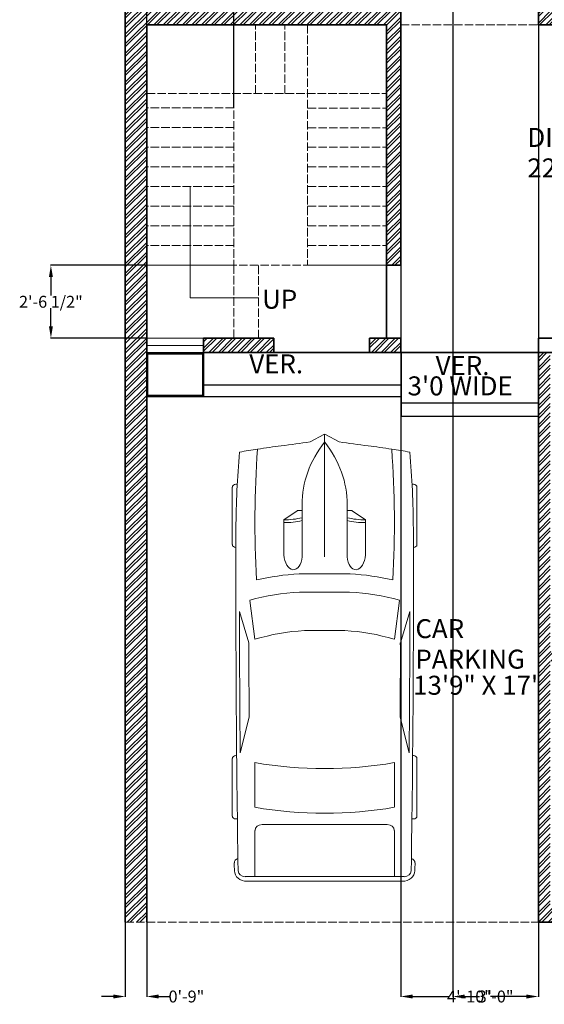
# Model space of a CAD drawing. Units: inches. Extents: x 334 to 846, y -424 to 250.
# Tile 1 of 3: x 336 to 557, y -420 to -5. Entities that reach past the tile are written whole.
import ezdxf

# ---------------------------------------------------------------- set-up
doc = ezdxf.new("R2010")
doc.units = ezdxf.units.IN
doc.header["$MEASUREMENT"] = 0
doc.linetypes.add('ACAD_ISO02W100', pattern=[15, 12, -3])
for name, color, linetype, lineweight in [('A-ANNO-SYMB', 7, 'Continuous', 18), ('A-ANNO-TEXT', 130, 'Continuous', 18), ('A-AREA-IDEN', 130, 'Continuous', 18), ('A-FLOR', 7, 'Continuous', 25), ('A-FLOR-STRS', 7, 'ACAD_ISO02W100', 18), ('A-WALL', 7, 'Continuous', 35), ('A-WALL-OVHD', 8, 'ACAD_ISO02W100', 18), ('A-WALL-PATT', 252, 'Continuous', 13), ('C-PRKG-VEHC', 8, 'Continuous', 18), ('C-PROP', 7, 'ACAD_ISO02W100', 18), ('dimension', 130, 'Continuous', 18), ('window', 150, 'Continuous', 18)]:
    doc.layers.add(name, color=color, linetype=linetype, lineweight=lineweight)
doc.styles.get("Standard").update_dxf_attribs({"font": 'arial.ttf'})
doc.dimstyles.get("Standard").update_dxf_attribs({"dimtxt": 5, "dimasz": 5, "dimexe": 0.18, "dimexo": 0.0625, "dimgap": 0.09, "dimtad": 0, "dimtih": 1, "dimtoh": 1, "dimdec": 1, "dimzin": 0, "dimdsep": 46, "dimlunit": 4, "dimtxsty": 'Standard', "dimcen": 0.09, "dimadec": 0, "dimazin": 0, "dimtfac": 1, "dimtdec": 1, "dimtofl": 0, "dimtmove": 0, "dimatfit": 3, "dimfxl": 1, "dimtolj": 1, "dimtzin": 0, "dimarcsym": 0})

# ---------------------------------------------------------------- blocks, each defined once
blk = doc.blocks.new('*U6')
for p, q in [((536, 950), (536, 936)), ((1182, 988), (568, 988)), ((1214, 950), (1214, 950)), ((3440, 942), (3440, 950)), ((3472, 988), (4087, 988)), ((4119, 950), (4119, 934)), ((2235, 810), (1899, 912)), ((3412, 904), (3030, 807)), ((4736, -851), (4736, 851)), ((1779, 801), (2195, 746)), ((3516, 746), (3994, 746)), ((4736, 746), (4242, 746)), ((4785, -832), (4785, 832)), ((4179, 670), (4179, -670)), ((820, 295), (918, 436)), ((918, 436), (1294, 436)), ((756, 241), (1313, 241)), ((816, 241), (816, 283)), ((1496, -274), (1496, 274)), ((1690, -267), (1690, 267)), ((2102, 216), (2102, -216)), ((4736, -267), (4736, 267)), ((83, 156), (3, 10)), ((0, 0), (1313, 0)), ((3, -10), (83, -156)), ((756, -241), (1313, -241)), ((816, -241), (816, -283)), ((820, -295), (918, -436)), ((918, -436), (1294, -436)), ((2195, -746), (1779, -801)), ((2235, -810), (1899, -912)), ((3412, -904), (3030, -807)), ((3994, -746), (3516, -746)), ((4242, -746), (4736, -746)), ((536, -950), (536, -936)), ((3440, -942), (3440, -950)), ((4119, -950), (4119, -934)), ((1182, -988), (568, -988)), ((1214, -950), (1214, -950)), ((3472, -988), (4087, -988))]:
    blk.add_line(p, q)
for centre, major_axis, ratio, start_param, end_param in [((1046, -12468), (0, 13417), 0.842304, 0.00281, 0.075598), ((568, 950), (0, -37.6), 0.842304, 3.141593, 4.712389), ((1638, -268113), (0, 269063), 0.842304, -0.013397, 0.002797), ((1182, 950), (0, 37.6), 0.842304, -1.570796, 0), ((3472, 950), (0, -37.6), 0.842304, 3.141593, 4.712389), ((4087, 950), (0, 37.6), 0.842304, -1.570796, 0), ((4588, 910), (0, 56.4), 0.842304, -0.013017, 1.249894), ((1638, -268131), (0, 269121), 0.842304, -0.013397, -0.013017), ((4673, 832), (0, -133), 0.842304, 1.570796, 3.128196), ((6757, -699), (0, 7958), 0.842304, 1.367076, 1.39176), ((1638, -268113), (0, -269025), 0.842304, 3.133765, 3.140441), ((4673, 851), (0, -75.2), 0.842304, 1.570796, 3.128196), ((952, -15087), (0, -15833), 0.842304, 3.096046, 3.200911), ((3436, 137), (0, 2077), 0.842304, 1.245306, 1.50788), ((3800, 71), (0, -2021), 0.842304, 4.372215, 4.640744), ((2433, -93125), (0, -93935), 0.842304, 3.134049, 3.144098), ((434, 0), (0, 3734), 0.842304, 4.511394, 4.913384), ((912, 0), (0, 3734), 0.842304, 4.511394, 4.913384), ((4242, 670), (0, 75.2), 0.842304, 0, 1.570796), ((6583, -699), (0, -7755), 0.842304, 4.528606, 4.561838), ((3414, 137), (0, -2280), 0.842304, 4.449482, 4.652344), ((-5194, 1331), (0, -6374), 0.842304, 1.385369, 1.434372), ((331, 432), (0, 696), 0.842304, 4.435146, 4.718221), ((361, 432), (0, 696), 0.842304, 4.435146, 4.718221), ((1290, 339), (161, -9), 0.603834, -1.395552, 1.581315), ((756, -1185), (0, 1427), 0.842304, 0, 0.590319), ((832, 283), (0, 18.8), 0.842304, 0.879714, 1.570796), ((16, 0), (0, -18.8), 0.842304, 4.131459, 5.293319), ((756, 1185), (0, 1427), 0.842304, 2.551274, 3.141593), ((-5194, -1331), (0, 6374), 0.842304, -1.434372, -1.385369), ((832, -283), (0, -18.8), 0.842304, 4.712389, 5.403472), ((331, -432), (0, -696), 0.842304, 1.564964, 1.848039), ((361, -432), (0, -696), 0.842304, 1.564964, 1.848039), ((3414, -137), (0, -2280), 0.842304, -1.510751, -1.307889), ((3436, -137), (0, -2077), 0.842304, -1.50788, -1.245306), ((3800, -71), (0, -2021), 0.842304, -1.499151, -1.230623), ((6583, 699), (0, 7755), 0.842304, 1.721348, 1.754579), ((6757, 699), (0, 7958), 0.842304, 1.749832, 1.774517), ((952, 15087), (0, -15833), 0.842304, -0.059319, 0.045547), ((4242, -670), (0, -75.2), 0.842304, 4.712389, 6.283185), ((2433, 93125), (0, -93935), 0.842304, -0.002505, 0.007544), ((4673, -832), (0, -133), 0.842304, 0.013397, 1.570796), ((1046, 12468), (0, -13417), 0.842304, -0.075598, -0.00281), ((1638, 268113), (0, 269063), 0.842304, 3.138796, 3.15499), ((1638, 268113), (0, -269025), 0.842304, 0.001152, 0.007828), ((4588, -910), (0, -56.4), 0.842304, -1.249894, 0.013017), ((4673, -851), (0, 75.2), 0.842304, 3.15499, 4.712389), ((568, -950), (0, 37.6), 0.842304, 1.570796, 3.141593), ((1182, -950), (0, -37.6), 0.842304, 0, 1.570796), ((3472, -950), (0, -37.6), 0.842304, -1.570796, 0), ((4087, -950), (0, 37.6), 0.842304, 3.141593, 4.712389), ((1638, 268131), (0, 269121), 0.842304, 3.15461, 3.15499)]:
    blk.add_ellipse(centre, major_axis=major_axis, ratio=ratio, start_param=start_param, end_param=end_param)
at = {"extrusion": (0, 0, -1)}
blk.add_ellipse((1290, -339), major_axis=(161, 9), ratio=0.603834, start_param=-1.395552, end_param=1.581315, dxfattribs=at)
blk = doc.blocks.new('*D23')
at = {"layer": 'Defpoints', "color": 0, "ltscale": 0.3, "transparency": 16777216}
for p in [(518.06, 70), (554.06, 65), (554.06, -416.35)]:
    blk.add_point(p, dxfattribs=at)
at = {"layer": 'dimension', "color": 0, "lineweight": -2, "ltscale": 0.3, "transparency": 16777216}
for p, q in [((518.06, 69.93), (518.06, -416.53)), ((554.06, 64.93), (554.06, -416.53)), ((523.06, -416.35), (529.33, -416.35)), ((549.06, -416.35), (542.8, -416.35))]:
    blk.add_line(p, q, dxfattribs=at)
at = {"layer": 'dimension', "color": 0, "ltscale": 0.3, "transparency": 16777216}
for points in [[(523.06, -415.52), (523.06, -417.19), (518.06, -416.35)], [(549.06, -415.52), (549.06, -417.19), (554.06, -416.35)]]:
    blk.add_solid(points, dxfattribs=at)
at = {"layer": 'dimension', "color": 0, "ltscale": 0.3, "transparency": 16777216, "insert": (536.06, -416.35), "char_height": 5, "attachment_point": 5}
blk.add_mtext('\\A1;3\'-0"', dxfattribs=at)
blk = doc.blocks.new('*D27')
at = {"layer": 'Defpoints', "color": 0, "ltscale": 0.3, "transparency": 16777216}
for p in [(496.06, -7), (554.06, -7), (554.06, -416.35)]:
    blk.add_point(p, dxfattribs=at)
at = {"layer": 'dimension', "color": 0, "lineweight": -2, "ltscale": 0.3, "transparency": 16777216}
for p, q in [((496.06, -7.07), (496.06, -416.53)), ((554.06, -7.07), (554.06, -416.53)), ((501.06, -416.35), (516.28, -416.35)), ((549.06, -416.35), (533.84, -416.35))]:
    blk.add_line(p, q, dxfattribs=at)
at = {"layer": 'dimension', "color": 0, "ltscale": 0.3, "transparency": 16777216}
for points in [[(501.06, -415.52), (501.06, -417.19), (496.06, -416.35)], [(549.06, -415.52), (549.06, -417.19), (554.06, -416.35)]]:
    blk.add_solid(points, dxfattribs=at)
at = {"layer": 'dimension', "color": 0, "ltscale": 0.3, "transparency": 16777216, "insert": (525.06, -416.35), "char_height": 5, "attachment_point": 5}
blk.add_mtext('\\A1;4\'-10"', dxfattribs=at)
blk = doc.blocks.new('*D31')
at = {"layer": 'Defpoints', "color": 0, "ltscale": 0.3, "transparency": 16777216}
for p in [(425.8, 242.35), (389.06, -35.92), (425.8, -41.92)]:
    blk.add_point(p, dxfattribs=at)
at = {"layer": 'dimension', "color": 0, "lineweight": -2, "ltscale": 0.3, "transparency": 16777216}
for p, q in [((389.06, -35.86), (389.06, 242.53)), ((394.06, 242.35), (394.87, 242.35)), ((420.8, 242.35), (419.99, 242.35)), ((425.8, -41.86), (425.8, 242.53))]:
    blk.add_line(p, q, dxfattribs=at)
at = {"layer": 'dimension', "color": 0, "ltscale": 0.3, "transparency": 16777216}
for points in [[(394.06, 243.18), (394.06, 241.51), (389.06, 242.35)], [(420.8, 243.18), (420.8, 241.51), (425.8, 242.35)]]:
    blk.add_solid(points, dxfattribs=at)
at = {"layer": 'dimension', "color": 0, "ltscale": 0.3, "transparency": 16777216, "insert": (407.43, 242.35), "char_height": 5, "attachment_point": 5}
blk.add_mtext('\\A1;3\'-0 1/2"', dxfattribs=at)
blk = doc.blocks.new('*D32')
at = {"layer": 'Defpoints', "color": 0, "ltscale": 0.3, "transparency": 16777216}
for p in [(389.06, -108.26), (348.71, -139), (389.06, -139)]:
    blk.add_point(p, dxfattribs=at)
at = {"layer": 'dimension', "color": 0, "lineweight": -2, "ltscale": 0.3, "transparency": 16777216}
for p, q in [((389, -108.26), (348.53, -108.26)), ((348.71, -113.26), (348.71, -120.96)), ((348.71, -134), (348.71, -126.31)), ((389, -139), (348.53, -139))]:
    blk.add_line(p, q, dxfattribs=at)
at = {"layer": 'dimension', "color": 0, "ltscale": 0.3, "transparency": 16777216}
for points in [[(347.88, -113.26), (349.55, -113.26), (348.71, -108.26)], [(347.88, -134), (349.55, -134), (348.71, -139)]]:
    blk.add_solid(points, dxfattribs=at)
at = {"layer": 'dimension', "color": 0, "ltscale": 0.3, "transparency": 16777216, "insert": (348.71, -123.63), "char_height": 5, "attachment_point": 5}
blk.add_mtext('\\A1;2\'-6 1/2"', dxfattribs=at)
blk = doc.blocks.new('*D33')
at = {"layer": 'Defpoints', "color": 0, "ltscale": 0.3, "transparency": 16777216}
for p in [(380.06, -385), (389.06, -385), (389.06, -416.35)]:
    blk.add_point(p, dxfattribs=at)
at = {"layer": 'dimension', "color": 0, "lineweight": -2, "ltscale": 0.3, "transparency": 16777216}
for p, q in [((380.06, -385.07), (380.06, -416.53)), ((389.06, -385.07), (389.06, -416.53)), ((375.06, -416.35), (370.06, -416.35)), ((394.06, -416.35), (399.06, -416.35))]:
    blk.add_line(p, q, dxfattribs=at)
at = {"layer": 'dimension', "color": 0, "ltscale": 0.3, "transparency": 16777216}
for points in [[(375.06, -415.52), (375.06, -417.19), (380.06, -416.35)], [(394.06, -415.52), (394.06, -417.19), (389.06, -416.35)]]:
    blk.add_solid(points, dxfattribs=at)
at = {"layer": 'dimension', "color": 0, "ltscale": 0.3, "transparency": 16777216, "insert": (405.8, -416.35), "char_height": 5, "attachment_point": 5}
blk.add_mtext('\\A1;0\'-9"', dxfattribs=at)

msp = doc.modelspace()

# ---------------------------------------------------------------- hatches: boundary and pattern name
at = {"layer": 'A-WALL-PATT', "ltscale": 0.3}
h = msp.add_hatch(dxfattribs=at)
h.set_pattern_fill('ANSI32', color=256, scale=7.6)
h.paths.add_polyline_path([(559.06, 149), (633.1, 149), (633.1, 154), (559.06, 154), (554.06, 154), (554.06, 33.31), (559.06, 33.31)], flags=17)
h.paths.add_polyline_path([(777.06, 211), (380.06, 211), (380.06, -385), (389.06, -385), (389.06, -7), (490.06, -7), (490.06, -108.26), (496.06, -108.26), (496.06, -7), (496.06, -1), (389.06, -1), (389.06, 65), (493.06, 65), (493.06, 33.31), (496.06, 33.31), (496.06, 65), (518.06, 65), (518.06, 70), (389.06, 70), (389.06, 202), (554.06, 202), (562.49, 202), (768.06, 202), (768.06, 154), (721.47, 154), (721.47, 149), (768.06, 149), (768.06, -1), (702.06, -1), (702.06, 19.69), (697.06, 19.69), (697.06, -1), (554.06, -1), (554.06, -7), (697.06, -7), (768.06, -7), (768.06, -145), (702.06, -145), (697.06, -145), (666.86, -145), (666.86, -151), (697.06, -151), (702.06, -151), (768.06, -151), (768.06, -205), (735.06, -205), (735.06, -211), (768.06, -211), (768.06, -271), (758.48, -271), (758.48, -275), (768.06, -275), (768.06, -349), (768.06, -379), (702.06, -379), (697.06, -379), (559.06, -379), (559.06, -349), (559.06, -275), (566.23, -275), (566.23, -271), (559.06, -271), (559.06, -145), (554.06, -145), (554.06, -349), (554.06, -385), (559.06, -385), (697.06, -385), (702.06, -385), (768.06, -385), (777.06, -385), (777.06, -349)])
h = msp.add_hatch(dxfattribs=at)
h.set_pattern_fill('ANSI32', color=256, scale=7.6)
h.paths.add_polyline_path([(702.06, 154), (687.41, 154), (687.41, 149), (697.06, 149), (697.06, 56.25), (702.06, 56.25)], flags=17)
h.paths.add_polyline_path([(442.56, -139), (413.06, -139), (413.06, -145), (442.56, -145)], flags=17)
h.paths.add_polyline_path([(496.06, -139), (482.97, -139), (482.97, -145), (496.06, -145)], flags=17)
h.paths.add_polyline_path([(702.98, -271), (668.71, -271), (642.67, -271), (621.73, -271), (621.73, -275), (642.67, -275), (679.56, -275), (702.98, -275)], flags=17)
h.paths.add_polyline_path([(768.06, 63), (729.58, 63), (729.58, 59), (747.32, 59), (768.06, 59)], flags=17)

# ---------------------------------------------------------------- linework, layer by layer
at = {"layer": 'A-ANNO-SYMB', "ltscale": 0.3}
for p, q in [((407.43, -75.06), (407.43, -108.26)), ((407.43, -108.26), (407.43, -121.98)), ((407.43, -121.98), (425.8, -121.98)), ((425.8, -121.98), (436.14, -121.98))]:
    msp.add_line(p, q, dxfattribs=at)
at = {"layer": 'A-FLOR', "ltscale": 0.3}
for p, q in [((413.06, -158.66), (496.31, -158.66)), ((496.31, -166.24), (554.06, -166.24))]:
    msp.add_line(p, q, dxfattribs=at)
for points in [[(389.06, -145), (413.06, -145), (413.06, -163.66), (389.06, -163.66)], [(413.06, -145), (496.31, -145), (496.31, -163.66), (413.06, -163.66)], [(554.06, -145), (496.31, -145), (496.31, -171.85), (554.06, -171.85)], [(389.56, -145.5), (412.56, -145.5), (412.56, -163.16), (389.56, -163.16)]]:
    msp.add_lwpolyline(points, close=True, dxfattribs=at)
at = {"layer": 'A-FLOR-STRS', "ltscale": 0.3}
for p, q in [((425.8, -7), (425.8, -108.26)), ((434.94, -35.92), (434.94, -7)), ((447.19, -35.92), (447.19, -7)), ((456.87, -7), (456.87, -108.26)), ((389.06, -35.92), (490.06, -35.92)), ((425.8, -41.92), (389.06, -41.92)), ((456.87, -41.99), (490.06, -41.99)), ((425.8, -50.21), (389.06, -50.21)), ((456.87, -50.28), (490.06, -50.28)), ((425.8, -58.49), (389.06, -58.49)), ((456.87, -58.56), (490.06, -58.56)), ((425.8, -66.77), (389.06, -66.77)), ((456.87, -66.84), (490.06, -66.84)), ((425.8, -75.06), (389.06, -75.06)), ((456.87, -75.13), (490.06, -75.13)), ((425.8, -83.34), (389.06, -83.34)), ((456.87, -83.41), (490.06, -83.41)), ((425.8, -91.62), (389.06, -91.62)), ((456.87, -91.69), (490.06, -91.69)), ((425.8, -99.91), (389.06, -99.91)), ((456.87, -99.98), (490.06, -99.98)), ((425.8, -108.19), (389.06, -108.19)), ((490.06, -108.26), (389.06, -108.26)), ((425.8, -108.26), (425.8, -139)), ((436.14, -139), (436.14, -108.26)), ((456.87, -108.26), (490.06, -108.26))]:
    msp.add_line(p, q, dxfattribs=at)
at = {"layer": 'A-WALL'}
for p, q in [((554.06, 154), (554.06, -7)), ((496.06, -1), (496.06, -7)), ((496.06, -7), (496.06, -108.26))]:
    msp.add_line(p, q, dxfattribs=at)
at = {"layer": 'A-WALL', "ltscale": 0.3}
msp.add_line((490.06, -108.26), (496.06, -108.26), dxfattribs=at)
for points in [[(554.06, -385), (559.06, -385), (697.06, -385), (702.06, -385), (768.06, -385), (777.06, -385), (777.06, -349), (777.06, 211), (380.06, 211), (380.06, -385)], [(666.86, -145), (697.06, -145), (702.06, -145), (768.06, -145), (768.06, -7), (697.06, -7), (554.06, -7)], [(413.06, -145), (442.56, -145), (442.56, -139), (413.06, -139), (413.06, -145), (496.06, -145), (554.06, -145), (554.06, -349), (554.06, -385)], [(496.06, -145), (496.06, -139), (482.97, -139), (482.97, -145)], [(554.06, -145), (559.06, -145), (567.61, -145)]]:
    msp.add_lwpolyline(points, dxfattribs=at)
at = {"layer": 'A-WALL'}
msp.add_lwpolyline([(389.06, -385), (389.06, -7), (490.06, -7), (490.06, -139)], dxfattribs=at)
at = {"layer": 'A-WALL', "ltscale": 0.3}
msp.add_lwpolyline([(554.06, -139), (567.61, -139), (567.61, -145), (554.06, -145)], close=True, dxfattribs=at)
at = {"layer": 'A-WALL-OVHD', "ltscale": 0.3}
msp.add_line((496.06, -7), (554.06, -7), dxfattribs=at)
at = {"layer": 'C-PROP', "ltscale": 0.3}
for p, q in [((380.06, -385), (389.06, -385)), ((389.06, -385), (554.06, -385))]:
    msp.add_line(p, q, dxfattribs=at)
at = {"layer": 'window', "ltscale": 0.3}
msp.add_line((389.06, -142), (413.06, -142), dxfattribs=at)
msp.add_lwpolyline([(389.06, -139), (413.06, -139), (413.06, -145), (389.06, -145)], close=True, dxfattribs=at)

# ---------------------------------------------------------------- block references
at = {"layer": 'C-PRKG-VEHC', "xscale": 0.0393700787401575, "yscale": 0.0393700787401575, "zscale": 0.0393700787401575, "rotation": 270}
msp.add_blockref('*U6', (464.03, -179.39), dxfattribs=at)

# ---------------------------------------------------------------- texts
at = {"layer": 'A-ANNO-TEXT', "ltscale": 0.3}
msp.add_text('UP', height=8, dxfattribs=at).set_placement((437.7, -126.56))
at = {"layer": 'A-AREA-IDEN', "ltscale": 0.3}
for s, p in [('DINING HALL', (549.43, -58.39)), ('22\'7" X 11\'6"', (549.43, -71.24)), ('VER.', (432.29, -153.79)), ('VER.', (510.79, -154.49)), ("3'0 WIDE", (498.96, -163.08)), ('CAR', (502.26, -265.36)), ('PARKING ', (502.26, -278.21)), ('13\'9" X 17\'', (501.3, -289.21))]:
    msp.add_text(s, height=8, dxfattribs=at).set_placement(p)

# ---------------------------------------------------------------- dimensions: what is measured, and where the dimension line sits
at = {"layer": 'dimension', "ltscale": 0.3}
for base, p1, p2, picture, middle in [((425.8, 242.35), (389.06, -35.92), (425.8, -41.92), '*D31', (407.43, 242.35)), ((554.06, -416.35), (518.06, 70), (554.06, 65), '*D23', (536.06, -416.35)), ((554.06, -416.35), (496.06, -7), (554.06, -7), '*D27', (525.06, -416.35)), ((389.06, -416.35), (380.06, -385), (389.06, -385), '*D33', (405.8, -416.35))]:
    dim = msp.add_linear_dim(base=base, p1=p1, p2=p2, dimstyle='Standard', override={"dimdec": 1, "dimlfac": 1, "dimrnd": 0, "dimzin": 1, "dimdsep": 46, "dimlunit": 4, "dimfrac": 2}, dxfattribs=at)
    dim.commit()
    dim.dimension.update_dxf_attribs({"geometry": picture, "text_midpoint": middle})
dim = msp.add_linear_dim(base=(348.71, -139), p1=(389.06, -108.26), p2=(389.06, -139), angle=90, dimstyle='Standard', override={"dimdec": 1, "dimlfac": 1, "dimrnd": 0, "dimzin": 1, "dimdsep": 46, "dimlunit": 4, "dimfrac": 2}, dxfattribs=at)
dim.commit()
dim.dimension.update_dxf_attribs({"geometry": '*D32', "text_midpoint": (348.71, -123.63)})

doc.saveas('drawing.dxf')
